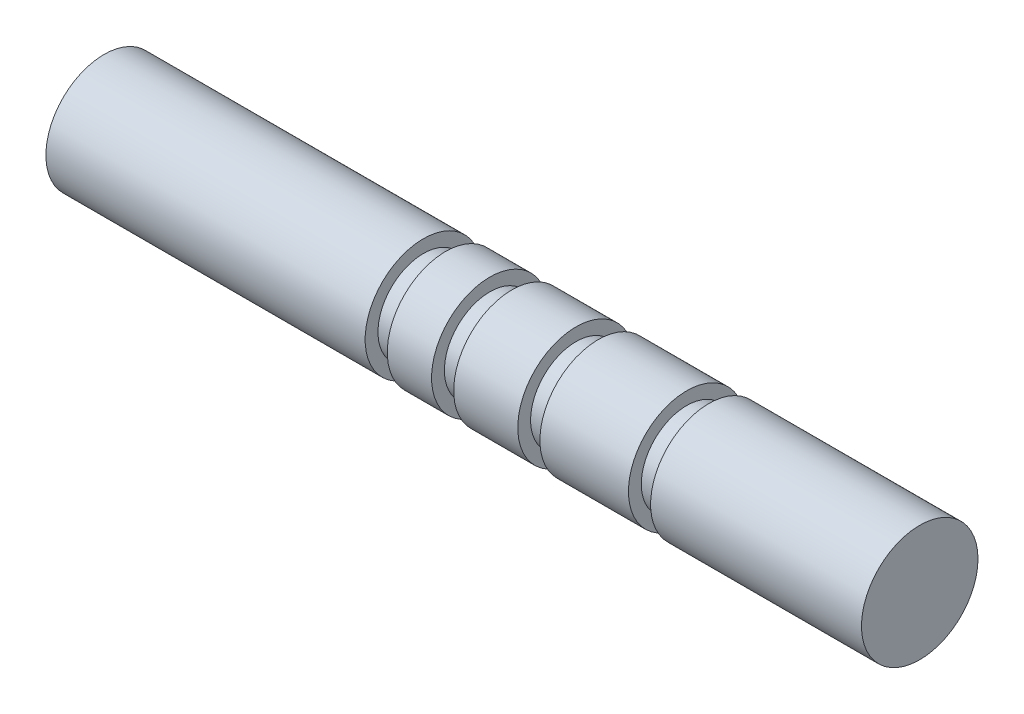
SolidWorks part; units mm, degrees
material "Plain Carbon Steel"
ref_plane "Front Plane" through (0, 0, 0) normal (0, 0, 1) x (1, 0, 0)
ref_plane "Top Plane" through (0, 0, 0) normal (0, 1, 0) x (1, 0, 0)
ref_plane "Right Plane" through (0, 0, 0) normal (1, 0, 0) x (0, 0, -1)
sketch "Rod Half-Profile Sketch" plane through (0, 0, 0) normal (0, 0, 1) x (1, 0, 0)
  line L0 (49.9914, 0) -> (-56.4265, 0) construction
  line L1 (-44.45, 0) -> (-44.45, 6.35)
  line L2 (-44.45, 6.35) -> (-9.652, 6.35)
  line L3 (-9.652, 6.35) -> (-9.652, 4.953)
  line L4 (-9.652, 4.953) -> (-7.239, 4.953)
  line L5 (-7.239, 4.953) -> (-7.239, 6.35)
  line L6 (-7.239, 6.35) -> (-2.413, 6.35)
  line L7 (-2.413, 6.35) -> (-2.413, 4.953)
  line L8 (-2.413, 4.953) -> (0, 4.953)
  line L9 (0, 4.953) -> (0, 6.35)
  line L10 (0, 6.35) -> (6.985, 6.35)
  line L11 (6.985, 6.35) -> (6.985, 4.953)
  line L12 (6.985, 4.953) -> (9.398, 4.953)
  line L13 (9.398, 4.953) -> (9.398, 6.35)
  line L14 (9.398, 6.35) -> (19.05, 6.35)
  line L15 (19.05, 6.35) -> (19.05, 4.953)
  line L16 (19.05, 4.953) -> (21.463, 4.953)
  line L17 (21.463, 4.953) -> (21.463, 6.35)
  line L18 (21.463, 6.35) -> (44.45, 6.35)
  line L19 (44.45, 6.35) -> (44.45, 0)
  line L20 (-44.45, 0) -> (44.45, 0)
  dimension "D1" = 88.9
  dimension "D2" = 25.4
  dimension "D3" = 2.413
  dimension "D4" = 35.052
  dimension "D5" = 44.45
  dimension "D6" = 54.102
  dimension "D7" = 6.35
  dimension "0.39/2" = 4.953
revolve "Grooved Rod Revolve" add sketch "Rod Half-Profile Sketch" angle 360 about L0
